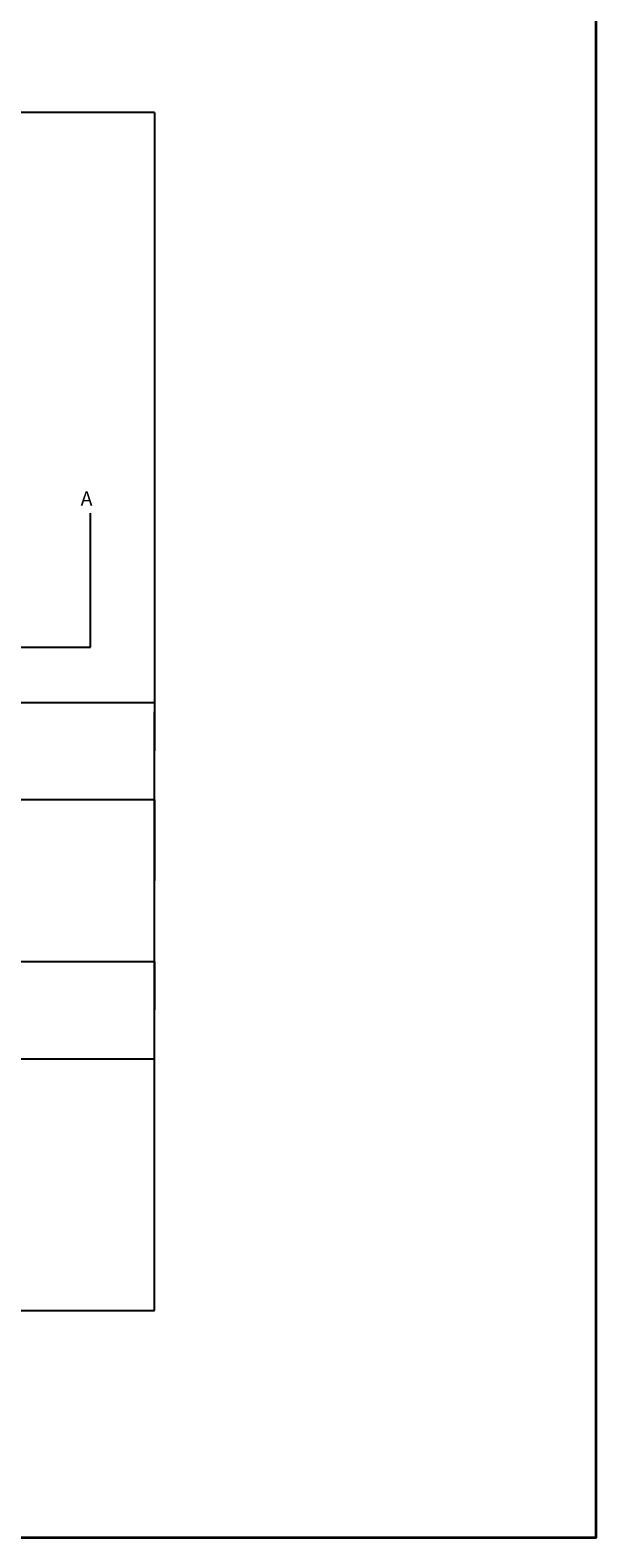
# Model space of a CAD drawing. Units: inches. Extents: x 2185 to 4426, y 1138 to 3073.
# Tile 13 of 14: x 3955 to 4426, y 1138 to 2395. Entities that reach past the tile are written whole.
import ezdxf

# ---------------------------------------------------------------- set-up
doc = ezdxf.new("R2010")
doc.units = ezdxf.units.IN
for name, color, linetype, lineweight in [('A-ANNO-DIMS', 2, 'Continuous', 18), ('A-ANNO-SYMB', 2, 'Continuous', 25), ('A-ANNO-TTLB', 7, 'Continuous', 35)]:
    doc.layers.add(name, color=color, linetype=linetype, lineweight=lineweight)
doc.styles.get("Standard").update_dxf_attribs({"font": 'arial.ttf'})
doc.dimstyles.get("Standard").update_dxf_attribs({"dimtxt": 0.18, "dimasz": 0.18, "dimexe": 0.18, "dimexo": 0.0625, "dimgap": 0.09, "dimtad": 0, "dimtih": 1, "dimtoh": 1, "dimdec": 4, "dimzin": 0, "dimdsep": 46, "dimtxsty": 'Standard', "dimcen": 0.09, "dimadec": 0, "dimazin": 0, "dimtfac": 1, "dimtdec": 4, "dimtofl": 0, "dimtmove": 0, "dimatfit": 3, "dimfxl": 1, "dimtolj": 1, "dimtzin": 0, "dimarcsym": 0})

# ---------------------------------------------------------------- blocks, each defined once
blk = doc.blocks.new('*D146')
at = {"layer": 'A-ANNO-DIMS', "color": 0, "lineweight": -2, "transparency": 16777216}
for p, q in [((3932.4, 2326.4), (4058.6, 2326.4)), ((4058.5, 2326.2), (4058.5, 1827.1)), ((4058.5, 1327.6), (4058.5, 1826.7)), ((3932.4, 1327.4), (4058.6, 1327.4))]:
    blk.add_line(p, q, dxfattribs=at)
at = {"layer": 'A-ANNO-DIMS', "color": 0, "transparency": 16777216}
for points in [[(4058.4, 2326.2), (4058.5, 2326.2), (4058.5, 2326.4)], [(4058.4, 1327.6), (4058.5, 1327.6), (4058.5, 1327.4)]]:
    blk.add_solid(points, dxfattribs=at)
at = {"layer": 'Defpoints', "color": 0, "transparency": 16777216}
for p in [(3932.3, 2326.4), (4058.5, 2326.4), (3932.3, 1327.4)]:
    blk.add_point(p, dxfattribs=at)
at = {"layer": 'A-ANNO-DIMS', "color": 0, "transparency": 16777216, "insert": (4058.5, 1826.9), "char_height": 0.18, "attachment_point": 5}
blk.add_mtext('\\A1;999', dxfattribs=at)
blk = doc.blocks.new('*D158')
at = {"layer": 'A-ANNO-DIMS', "color": 0, "lineweight": -2, "transparency": 16777216}
for p, q in [((3665.4, 1618.4), (4058.6, 1618.4)), ((4058.5, 1618.2), (4058.5, 1578.1)), ((4058.5, 1537.6), (4058.5, 1577.7)), ((3746.4, 1537.4), (4058.6, 1537.4))]:
    blk.add_line(p, q, dxfattribs=at)
at = {"layer": 'A-ANNO-DIMS', "color": 0, "transparency": 16777216}
for points in [[(4058.4, 1618.2), (4058.5, 1618.2), (4058.5, 1618.4)], [(4058.4, 1537.6), (4058.5, 1537.6), (4058.5, 1537.4)]]:
    blk.add_solid(points, dxfattribs=at)
at = {"layer": 'Defpoints', "color": 0, "transparency": 16777216}
for p in [(3665.3, 1618.4), (4058.5, 1618.4), (3746.3, 1537.4)]:
    blk.add_point(p, dxfattribs=at)
at = {"layer": 'A-ANNO-DIMS', "color": 0, "transparency": 16777216, "insert": (4058.5, 1577.9), "char_height": 0.18, "attachment_point": 5}
blk.add_mtext('\\A1;81', dxfattribs=at)
blk = doc.blocks.new('*D159')
at = {"layer": 'A-ANNO-DIMS', "color": 0, "lineweight": -2, "transparency": 16777216}
for p, q in [((3665.4, 1753.4), (4058.6, 1753.4)), ((4058.5, 1753.2), (4058.5, 1686.1)), ((4058.5, 1618.6), (4058.5, 1685.7)), ((3665.4, 1618.4), (4058.6, 1618.4))]:
    blk.add_line(p, q, dxfattribs=at)
at = {"layer": 'A-ANNO-DIMS', "color": 0, "transparency": 16777216}
for points in [[(4058.4, 1753.2), (4058.5, 1753.2), (4058.5, 1753.4)], [(4058.4, 1618.6), (4058.5, 1618.6), (4058.5, 1618.4)]]:
    blk.add_solid(points, dxfattribs=at)
at = {"layer": 'Defpoints', "color": 0, "transparency": 16777216}
for p in [(3665.3, 1753.4), (4058.5, 1753.4), (3665.3, 1618.4)]:
    blk.add_point(p, dxfattribs=at)
at = {"layer": 'A-ANNO-DIMS', "color": 0, "transparency": 16777216, "insert": (4058.5, 1685.9), "char_height": 0.18, "attachment_point": 5}
blk.add_mtext('\\A1;135', dxfattribs=at)
blk = doc.blocks.new('*D160')
at = {"layer": 'A-ANNO-DIMS', "color": 0, "lineweight": -2, "transparency": 16777216}
for p, q in [((3746.4, 1834.4), (4058.6, 1834.4)), ((4058.5, 1834.2), (4058.5, 1794.1)), ((4058.5, 1753.6), (4058.5, 1793.7)), ((3665.4, 1753.4), (4058.6, 1753.4))]:
    blk.add_line(p, q, dxfattribs=at)
at = {"layer": 'A-ANNO-DIMS', "color": 0, "transparency": 16777216}
for points in [[(4058.4, 1834.2), (4058.5, 1834.2), (4058.5, 1834.4)], [(4058.4, 1753.6), (4058.5, 1753.6), (4058.5, 1753.4)]]:
    blk.add_solid(points, dxfattribs=at)
at = {"layer": 'Defpoints', "color": 0, "transparency": 16777216}
for p in [(3746.3, 1834.4), (4058.5, 1834.4), (3665.3, 1753.4)]:
    blk.add_point(p, dxfattribs=at)
at = {"layer": 'A-ANNO-DIMS', "color": 0, "transparency": 16777216, "insert": (4058.5, 1793.9), "char_height": 0.18, "attachment_point": 5}
blk.add_mtext('\\A1;81', dxfattribs=at)

msp = doc.modelspace()

# ---------------------------------------------------------------- linework, layer by layer
at = {"layer": 'A-ANNO-SYMB'}
for p, q in [((4005.21, 1880.563), (4005.21, 1992.352)), ((3155.074, 1880.563), (4005.21, 1880.563))]:
    msp.add_line(p, q, dxfattribs=at)
at = {"layer": 'A-ANNO-TTLB'}
msp.add_lwpolyline([(2184.741, 3073.364), (4426.252, 3073.364), (4426.252, 1137.99), (2184.741, 1137.99)], close=True, dxfattribs=at)

# ---------------------------------------------------------------- texts
at = {"layer": 'A-ANNO-SYMB', "insert": (3996.977, 2010.384), "char_height": 12, "attachment_point": 1}
msp.add_mtext_dynamic_manual_height_columns('A', width=59.61146, gutter_width=12.5, heights=[0], dxfattribs=at)

# ---------------------------------------------------------------- dimensions: what is measured, and where the dimension line sits
at = {"layer": 'A-ANNO-DIMS'}
for base, p1, p2, picture, middle in [((4058.46, 2326.377), (3932.349, 1327.377), (3932.349, 2326.377), '*D146', (4058.46, 1826.877)), ((4058.46, 1834.377), (3665.349, 1753.377), (3746.349, 1834.377), '*D160', (4058.46, 1793.877)), ((4058.46, 1753.377), (3665.349, 1618.377), (3665.349, 1753.377), '*D159', (4058.46, 1685.877)), ((4058.46, 1618.377), (3746.349, 1537.377), (3665.349, 1618.377), '*D158', (4058.46, 1577.877))]:
    dim = msp.add_linear_dim(base=base, p1=p1, p2=p2, angle=90, dimstyle='Standard', override={"dimdec": 0, "dimlfac": 1, "dimrnd": 0, "dimzin": 0, "dimdsep": 46, "dimlunit": 2}, dxfattribs=at)
    dim.commit()
    dim.dimension.update_dxf_attribs({"geometry": picture, "text_midpoint": middle})

doc.saveas('drawing.dxf')
